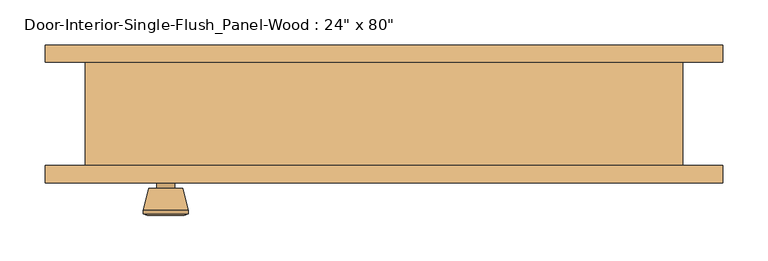
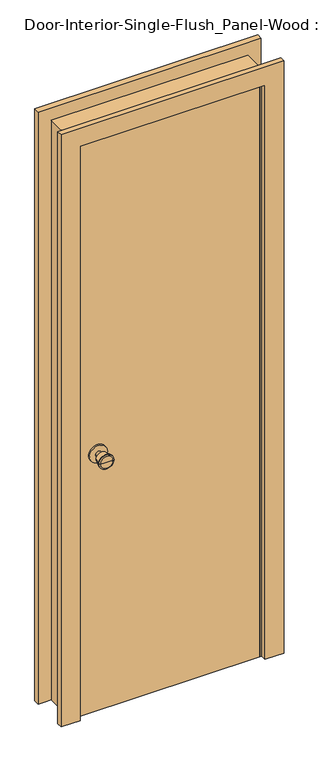
"""IFC4 building model written with IfcOpenShell, lengths in millimetres: door geometry."""

from ifc_helpers import new_model, si_unit, point, frame, frame_2d, origin, origin_with_axes, place, context, project, spatial, polyline, circle_curve, trimmed, segment, composite_curve, outline, extrude, faceted_brep, source, transform, mapped, element, save
from ifc_brep_helpers import plane_surface, cylinder_surface, revolved_surface, advanced_brep


def door_525aa856(model_context):
    return source(origin(), model_context, "Body", "SolidModel", [
        advanced_brep(
        [(-241.3, -13.05, 914.4), (-251.3, -13.05, 914.4), (-231.3, -13.05, 914.4), (-220.8241324, 35.95, 914.4), (-261.7758676, 35.95, 914.4), (-241.3, 35.95, 914.4), (-216.3, 34.1221319, 914.4), (-266.3, 34.1221319, 914.4), (-216.3, 30.6584537, 914.4), (-266.3, 30.6584537, 914.4), (-222.663764, 5.95, 914.4), (-259.936236, 5.95, 914.4), (-231.3, 5.95, 914.4), (-251.3, 5.95, 914.4)],
        [
            (0, 1),
            (1, 2, circle_curve(frame((-241.3, -13.05, 914.4), z_axis=(0.0, -1.0, 0.0), x_axis=(-1.0, 0.0, 0.0)), 10.0)),
            (2, 0),
            (2, 1, circle_curve(frame((-241.3, -13.05, 914.4), z_axis=(0.0, -1.0, 0.0), x_axis=(-1.0, 0.0, 0.0)), 10.0)),
            (3, 4, circle_curve(frame((-241.3, 35.95, 914.4), z_axis=(0.0, 1.0, 0.0), x_axis=(-1.0, 0.0, 0.0)), 20.4758676)),
            (4, 5),
            (5, 3),
            (4, 3, circle_curve(frame((-241.3, 35.95, 914.4), z_axis=(0.0, 1.0, 0.0), x_axis=(-1.0, 0.0, 0.0)), 20.4758676)),
            (6, 7, circle_curve(frame((-241.3, 34.1221319, 914.4), z_axis=(0.0, 1.0, 0.0), x_axis=(-1.0, 0.0, 0.0)), 25.0)),
            (7, 4),
            (3, 6),
            (7, 6, circle_curve(frame((-241.3, 34.1221319, 914.4), z_axis=(0.0, 1.0, 0.0), x_axis=(-1.0, 0.0, 0.0)), 25.0)),
            (8, 9, circle_curve(frame((-241.3, 30.6584537, 914.4), z_axis=(0.0, 1.0, 0.0), x_axis=(-1.0, 0.0, 0.0)), 25.0)),
            (9, 7),
            (6, 8),
            (9, 8, circle_curve(frame((-241.3, 30.6584537, 914.4), z_axis=(0.0, 1.0, 0.0), x_axis=(-1.0, 0.0, 0.0)), 25.0)),
            (10, 11, circle_curve(frame((-241.3, 5.95, 914.4), z_axis=(0.0, 1.0, 0.0), x_axis=(-1.0, 0.0, 0.0)), 18.636236)),
            (11, 9),
            (8, 10),
            (11, 10, circle_curve(frame((-241.3, 5.95, 914.4), z_axis=(0.0, 1.0, 0.0), x_axis=(-1.0, 0.0, 0.0)), 18.636236)),
            (12, 13, circle_curve(frame((-241.3, 5.95, 914.4), z_axis=(0.0, 1.0, 0.0), x_axis=(-1.0, 0.0, 0.0)), 10.0)),
            (13, 11),
            (10, 12),
            (13, 12, circle_curve(frame((-241.3, 5.95, 914.4), z_axis=(0.0, 1.0, 0.0), x_axis=(-1.0, 0.0, 0.0)), 10.0)),
            (1, 13),
            (12, 2),
        ],
        [
            plane_surface(frame((-241.3, -13.05, 914.4), z_axis=(0.0, -1.0, 0.0), x_axis=(-1.0, 0.0, 0.0))),
            plane_surface(frame((-241.3, 35.95, 914.4), z_axis=(0.0, 1.0, 0.0), x_axis=(-1.0, 0.0, 0.0))),
            revolved_surface(polyline([(-261.7758676, 35.95, 914.4), (-266.3, 34.1221319, 914.4)]), (-241.3, -13.05, 914.4), (0.0, -1.0, 0.0)),
            cylinder_surface(frame((-241.3, -13.05, 914.4), z_axis=(0.0, -1.0, 0.0), x_axis=(-1.0, 0.0, 0.0)), 25.0),
            revolved_surface(polyline([(-266.3, 30.6584537, 914.4), (-259.936236, 5.95, 914.4)]), (-241.3, -13.05, 914.4), (0.0, -1.0, 0.0)),
            plane_surface(frame((-241.3, 5.95, 914.4), z_axis=(0.0, -1.0, 0.0), x_axis=(-1.0, 0.0, 0.0))),
            cylinder_surface(frame((-241.3, -13.05, 914.4), z_axis=(0.0, -1.0, 0.0), x_axis=(-1.0, 0.0, 0.0)), 10.0),
        ],
        [
            (0, [[1, 2, 3]]),
            (0, [[-3, 4, -1]]),
            (1, [[5, 6, 7]]),
            (1, [[8, -7, -6]]),
            (2, [[9, 10, -5, 11]]),
            (2, [[12, -11, -8, -10]]),
            (3, [[13, 14, -9, 15]]),
            (3, [[16, -15, -12, -14]]),
            (4, [[17, 18, -13, 19]]),
            (4, [[20, -19, -16, -18]]),
            (5, [[21, 22, -17, 23]]),
            (5, [[24, -23, -20, -22]]),
            (6, [[-2, 25, -21, 26]]),
            (6, [[-4, -26, -24, -25]]),
        ],
    ),
        extrude(outline(composite_curve([segment(trimmed(circle_curve(frame_2d((914.4, -241.3)), 30.0), [point((914.4, -271.3))], [point((914.4, -211.3))], False, "CARTESIAN"), True, "CONTINUOUS"), segment(trimmed(circle_curve(frame_2d((914.4, -241.3)), 30.0), [point((914.4, -211.3))], [point((914.4, -271.3))], False, "CARTESIAN"), True, "CONTINUOUS")], self_intersect=False)), frame((0.0, -19.05, 0.0), z_axis=(0.0, 1.0, 0.0), x_axis=(0.0, 0.0, 1.0)), (0.0, 0.0, 1.0), 6.0),
        advanced_brep(
        [(-241.3, -59.975, 914.4), (-231.3, -59.975, 914.4), (-251.3, -59.975, 914.4), (-220.8241324, -108.975, 914.4), (-241.3, -108.975, 914.4), (-261.7758676, -108.975, 914.4), (-216.3, -107.1471319, 914.4), (-266.3, -107.1471319, 914.4), (-216.3, -103.6834537, 914.4), (-266.3, -103.6834537, 914.4), (-222.663764, -78.975, 914.4), (-259.936236, -78.975, 914.4), (-231.3, -78.975, 914.4), (-251.3, -78.975, 914.4)],
        [
            (0, 1),
            (1, 2, circle_curve(frame((-241.3, -59.975, 914.4), z_axis=(0.0, 1.0, 0.0), x_axis=(-1.0, 0.0, 0.0)), 10.0)),
            (2, 0),
            (2, 1, circle_curve(frame((-241.3, -59.975, 914.4), z_axis=(0.0, 1.0, 0.0), x_axis=(-1.0, 0.0, 0.0)), 10.0)),
            (3, 4),
            (4, 5),
            (5, 3, circle_curve(frame((-241.3, -108.975, 914.4), z_axis=(0.0, -1.0, 0.0), x_axis=(-1.0, 0.0, 0.0)), 20.4758676)),
            (3, 5, circle_curve(frame((-241.3, -108.975, 914.4), z_axis=(0.0, -1.0, 0.0), x_axis=(-1.0, 0.0, 0.0)), 20.4758676)),
            (6, 3),
            (5, 7),
            (7, 6, circle_curve(frame((-241.3, -107.1471319, 914.4), z_axis=(0.0, -1.0, 0.0), x_axis=(-1.0, 0.0, 0.0)), 25.0)),
            (6, 7, circle_curve(frame((-241.3, -107.1471319, 914.4), z_axis=(0.0, -1.0, 0.0), x_axis=(-1.0, 0.0, 0.0)), 25.0)),
            (8, 6),
            (7, 9),
            (9, 8, circle_curve(frame((-241.3, -103.6834537, 914.4), z_axis=(0.0, -1.0, 0.0), x_axis=(-1.0, 0.0, 0.0)), 25.0)),
            (8, 9, circle_curve(frame((-241.3, -103.6834537, 914.4), z_axis=(0.0, -1.0, 0.0), x_axis=(-1.0, 0.0, 0.0)), 25.0)),
            (10, 8),
            (9, 11),
            (11, 10, circle_curve(frame((-241.3, -78.975, 914.4), z_axis=(0.0, -1.0, 0.0), x_axis=(-1.0, 0.0, 0.0)), 18.636236)),
            (10, 11, circle_curve(frame((-241.3, -78.975, 914.4), z_axis=(0.0, -1.0, 0.0), x_axis=(-1.0, 0.0, 0.0)), 18.636236)),
            (12, 10),
            (11, 13),
            (13, 12, circle_curve(frame((-241.3, -78.975, 914.4), z_axis=(0.0, -1.0, 0.0), x_axis=(-1.0, 0.0, 0.0)), 10.0)),
            (12, 13, circle_curve(frame((-241.3, -78.975, 914.4), z_axis=(0.0, -1.0, 0.0), x_axis=(-1.0, 0.0, 0.0)), 10.0)),
            (1, 12),
            (13, 2),
        ],
        [
            plane_surface(frame((-241.3, -59.975, 914.4), z_axis=(0.0, 1.0, 0.0), x_axis=(-1.0, 0.0, 0.0))),
            plane_surface(frame((-241.3, -108.975, 914.4), z_axis=(0.0, -1.0, 0.0), x_axis=(-1.0, 0.0, 0.0))),
            revolved_surface(polyline([(-261.7758676, -108.975, 914.4), (-266.3, -107.1471319, 914.4)]), (-241.3, -59.975, 914.4), (0.0, 1.0, 0.0)),
            cylinder_surface(frame((-241.3, -59.975, 914.4), z_axis=(0.0, 1.0, 0.0), x_axis=(-1.0, 0.0, 0.0)), 25.0),
            revolved_surface(polyline([(-266.3, -103.6834537, 914.4), (-259.936236, -78.975, 914.4)]), (-241.3, -59.975, 914.4), (0.0, 1.0, 0.0)),
            plane_surface(frame((-241.3, -78.975, 914.4), z_axis=(0.0, 1.0, 0.0), x_axis=(-1.0, 0.0, 0.0))),
            cylinder_surface(frame((-241.3, -59.975, 914.4), z_axis=(0.0, 1.0, 0.0), x_axis=(-1.0, 0.0, 0.0)), 10.0),
        ],
        [
            (0, [[1, 2, 3]]),
            (0, [[-3, 4, -1]]),
            (1, [[5, 6, 7]]),
            (1, [[-6, -5, 8]]),
            (2, [[9, -7, 10, 11]]),
            (2, [[-10, -8, -9, 12]]),
            (3, [[13, -11, 14, 15]]),
            (3, [[-14, -12, -13, 16]]),
            (4, [[17, -15, 18, 19]]),
            (4, [[-18, -16, -17, 20]]),
            (5, [[21, -19, 22, 23]]),
            (5, [[-22, -20, -21, 24]]),
            (6, [[25, -23, 26, -2]]),
            (6, [[-26, -24, -25, -4]]),
        ],
    ),
        extrude(outline(composite_curve([segment(trimmed(circle_curve(frame_2d((914.4, -241.3)), 30.0), [point((914.4, -271.3))], [point((914.4, -211.3))], False, "CARTESIAN"), True, "CONTINUOUS"), segment(trimmed(circle_curve(frame_2d((914.4, -241.3)), 30.0), [point((914.4, -211.3))], [point((914.4, -271.3))], False, "CARTESIAN"), True, "CONTINUOUS")], self_intersect=False)), frame((0.0, -59.975, 0.0), z_axis=(0.0, 1.0, 0.0), x_axis=(0.0, 0.0, 1.0)), (0.0, 0.0, 1.0), 6.0),
        faceted_brep([(330.2, -53.975, 0.0), (304.8, -53.975, 0.0), (304.8, -19.05, 0.0), (292.1, -19.05, 0.0), (292.1, 15.875, 0.0), (304.8, 15.875, 0.0), (304.8, 60.325, 0.0), (330.2, 60.325, 0.0), (330.2, 60.325, 2057.4), (330.2, -53.975, 2057.4), (304.8, 60.325, 2032.0), (-304.8, 60.325, 2032.0), (-304.8, 60.325, 0.0), (-330.2, 60.325, 0.0), (-330.2, 60.325, 2057.4), (304.8, 15.875, 2032.0), (292.1, 15.875, 2019.3), (-292.1, 15.875, 2019.3), (-292.1, 15.875, 0.0), (-304.8, 15.875, 0.0), (-304.8, 15.875, 2032.0), (292.1, -19.05, 2019.3), (304.8, -19.05, 2032.0), (-304.8, -19.05, 2032.0), (-304.8, -19.05, 0.0), (-292.1, -19.05, 0.0), (-292.1, -19.05, 2019.3), (304.8, -53.975, 2032.0), (-330.2, -53.975, 2057.4), (-330.2, -53.975, 0.0), (-304.8, -53.975, 0.0), (-304.8, -53.975, 2032.0)], [[[0, 1, 2, 3, 4, 5, 6, 7]], [[7, 8, 9, 0]], [[6, 10, 11, 12, 13, 14, 8, 7]], [[5, 15, 10, 6]], [[4, 16, 17, 18, 19, 20, 15, 5]], [[3, 21, 16, 4]], [[2, 22, 23, 24, 25, 26, 21, 3]], [[1, 27, 22, 2]], [[0, 9, 28, 29, 30, 31, 27, 1]], [[8, 14, 28, 9]], [[15, 20, 11, 10]], [[21, 26, 17, 16]], [[27, 31, 23, 22]], [[29, 13, 12, 19, 18, 25, 24, 30]], [[14, 13, 29, 28]], [[20, 19, 12, 11]], [[26, 25, 18, 17]], [[31, 30, 24, 23]]]),
        extrude(outline(polyline([(304.8, -19.05), (304.8, -53.975), (-304.8, -53.975), (-304.8, -19.05), (304.8, -19.05)])), origin_with_axes(), (0.0, 0.0, 1.0), 2032.0),
        extrude(outline(polyline([(0.0, 374.65), (2101.85, 374.65), (2101.85, -374.65), (0.0, -374.65), (0.0, -311.15), (2038.35, -311.15), (2038.35, 311.15), (0.0, 311.15), (0.0, 374.65)])), frame((0.0, -73.025, 0.0), z_axis=(0.0, 1.0, 0.0), x_axis=(0.0, 0.0, 1.0)), (0.0, 0.0, 1.0), 19.05),
        extrude(outline(polyline([(0.0, 374.65), (2101.85, 374.65), (2101.85, -374.65), (0.0, -374.65), (0.0, -311.15), (2038.35, -311.15), (2038.35, 311.15), (0.0, 311.15), (0.0, 374.65)])), frame((0.0, 60.325, 0.0), z_axis=(0.0, 1.0, 0.0), x_axis=(0.0, 0.0, 1.0)), (0.0, 0.0, 1.0), 19.05),
    ])


if __name__ == "__main__":
    model = new_model("IFC4")
    model_context = context("Model", 3, world=origin())
    ifc_project = project(units=[si_unit("LENGTHUNIT", "METRE", prefix="MILLI")], contexts=[model_context])
    site = spatial("IfcSite", under=ifc_project)
    building = spatial("IfcBuilding", under=site)
    placement = place(None, origin())
    door_shape = door_525aa856(model_context)
    element("IfcDoor", 1, ObjectType="Door-Interior-Single-Flush_Panel-Wood : 24\" x 80\"", at=placement, inside=building, context=model_context, shape_type="MappedRepresentation", body=[
        mapped(door_shape, transform((0.0, 0.0, 0.0), x_axis=(1.0, 0.0, 0.0), y_axis=(0.0, 1.0, 0.0), z_axis=(0.0, 0.0, 1.0))),
    ])
    save(model, "model.ifc")

# Revit data of these elements
# Type "Door-Interior-Single-Flush_Panel-Wood : 24\" x 80\""
#   Type Mark = "12"
#   Assembly Code = "C1020300"
#   Analytic Construction = "Wooden"
#   Thickness = 0' - 1 3/8"
#   Thermal Resistance (R) = 2.5876 (h·ft²·°F)/BTU
#   Swing Angle [instance default] = 90.00°
#   Rough Width = 2' - 2"
#   Rough Height = 6' - 9"
#   Height = 6' - 8"
#   Width = 2' - 0"
#   Heat Transfer Coefficient (U) = 0.3865 BTU/(h·ft²·°F)
#   Trim Material = Cherry
#   Panel Material = Cherry
#   Frame Material = Cherry
#   Door Handle Material = Aluminum
#   Visual Light Transmittance = 0
#   Solar Heat Gain Coefficient = 0
#   Wall Closure = (empty or 0)
#   Function = (empty or 0)
# Element 1 (IfcDoor, "Door-Interior-Single-Flush_Panel-Wood : 24\" x 80\"")
#   Materials on its faces: "Cherry", "Aluminum"
# Materials
#   "Cherry": class "Wood", colour RGB 226 177 128, transparency 0, Description = "Prunus Serotina", Cost = 0
#   "Aluminum": class "Metal", colour RGB 247 247 247, transparency 0, Description = "Aluminum 6061", Cost = 0
